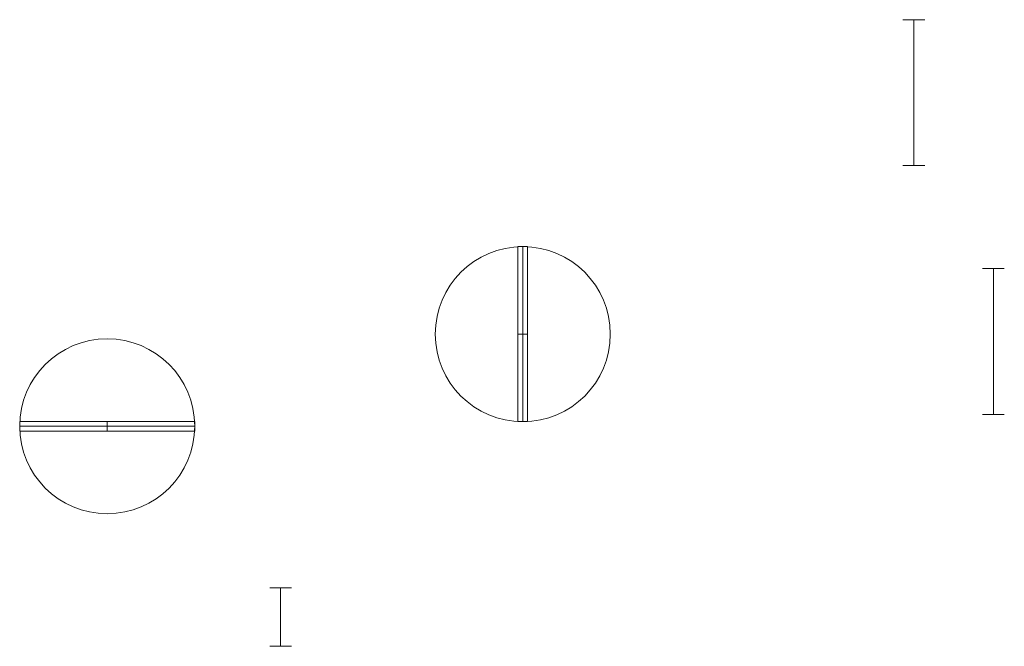
# Model space of a CAD drawing. Units: inches. Extents: x 774 to 2194, y 522 to 1247.
# Tile 7 of 7: x 1789 to 2194, y 749 to 1007. Entities that reach past the tile are written whole.
import ezdxf

# ---------------------------------------------------------------- set-up
doc = ezdxf.new("R2010")
doc.units = ezdxf.units.IN
doc.layers.add('A-DOOR', color=3, linetype='Continuous', lineweight=18)
doc.layers.add('A-GLAZ', color=4, linetype='Continuous', lineweight=18)

# ---------------------------------------------------------------- blocks, each defined once
blk = doc.blocks.new('DOOR-SWING-36IN')
blk.add_line((36, 0), (36, 2))
blk.add_lwpolyline([(36, 2), (0, 2), (0, 0), (36, 0)], close=True)
blk.add_arc((36, 0), 36, 90, 180)
blk = doc.blocks.new('WIN-60IN-EXT')
for p, q in [((0, 0), (0, 9)), ((60, 0), (60, 9)), ((0, 4.5), (60, 4.5))]:
    blk.add_line(p, q)
blk = doc.blocks.new('WIN-24IN-EXT')
for p, q in [((0, 0), (0, 9)), ((24, 0), (24, 9)), ((0, 4.5), (24, 4.5))]:
    blk.add_line(p, q)

msp = doc.modelspace()

# ---------------------------------------------------------------- block references
at = {"layer": 'A-DOOR', "extrusion": (0, 0, -1), "zscale": -1}
for p, rotation in [((-1995.83479, 913.67344), 270), ((-1995.83563, 841.67428), 90.00000000000003), ((-1788.89596, 839.76216), 180)]:
    msp.add_blockref('DOOR-SWING-36IN', p, dxfattribs=dict(at, rotation=rotation))
at = {"layer": 'A-DOOR'}
for p, rotation in [((1995.83563, 913.67344), 270), ((1995.83479, 841.67428), 90.00000000000003), ((1860.89512, 839.76216), 180)]:
    msp.add_blockref('DOOR-SWING-36IN', p, dxfattribs=dict(at, rotation=rotation))
msp.add_blockref('DOOR-SWING-36IN', (1788.89596, 839.76299), dxfattribs=at)
at = {"layer": 'A-DOOR', "extrusion": (0, 0, -1), "zscale": -1}
msp.add_blockref('DOOR-SWING-36IN', (-1860.89512, 839.76299), dxfattribs=at)
at = {"layer": 'A-GLAZ'}
for name, p, rotation in [('WIN-60IN-EXT', (2161.20099, 947.06789), 90.00000000000047), ('WIN-60IN-EXT', (2193.89532, 844.66448), 90.00000000000043), ('WIN-24IN-EXT', (1891.73638, 773.21955), 269.9999999999989)]:
    msp.add_blockref(name, p, dxfattribs=dict(at, rotation=rotation))

doc.saveas('drawing.dxf')
